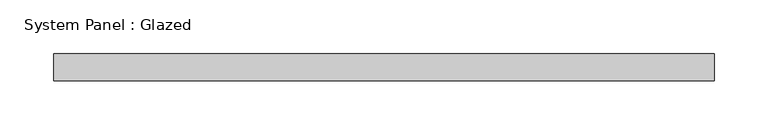
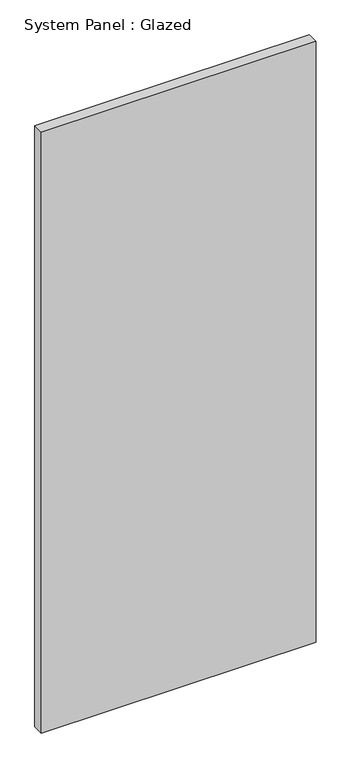
"""IFC4 building model written with IfcOpenShell, lengths in millimetres: plate geometry, System Panel : Glazed."""

from ifc_helpers import new_model, si_unit, origin, origin_with_axes, place, context, project, spatial, polyline, outline, extrude, source, transform, mapped, element, save


def system_panel_glazed_6c2109f1(model_context):
    return source(origin(), model_context, "Body", "SweptSolid", [
        extrude(outline(polyline([(307.975, 19.05), (-307.975, 19.05), (-307.975, 44.45), (307.975, 44.45), (307.975, 19.05)])), origin_with_axes(), (0.0, 0.0, 1.0), 1422.4),
    ])


if __name__ == "__main__":
    model = new_model("IFC4")
    model_context = context("Model", 3, world=origin())
    ifc_project = project(units=[si_unit("LENGTHUNIT", "METRE", prefix="MILLI")], contexts=[model_context])
    site = spatial("IfcSite", under=ifc_project)
    building = spatial("IfcBuilding", under=site)
    placement = place(None, origin())
    system_panel_glazed_shape = system_panel_glazed_6c2109f1(model_context)
    element("IfcPlate", 1, ObjectType="System Panel : Glazed", at=placement, inside=building, context=model_context, shape_type="MappedRepresentation", body=[
        mapped(system_panel_glazed_shape, transform((0.0, 0.0, 0.0), x_axis=(1.0, 0.0, 0.0), y_axis=(0.0, 1.0, 0.0), z_axis=(0.0, 0.0, 1.0))),
    ])
    save(model, "model.ifc")

# Revit data of these elements
# Type "System Panel : Glazed"
#   Construction Type Id = "GSP4R"
#   Analytic Construction = "1/8 in Pilkington single glazing"
#   Visual Light Transmittance = 0.9
#   Solar Heat Gain Coefficient = 0.86
#   Heat Transfer Coefficient (U) = 1.18115 BTU/(h·ft²·°F)
#   Define Thermal Properties by = 1
# Element 1 (IfcPlate, "System Panel : Glazed")
#   Materials on its faces: "Glass"
# Materials
#   "Glass": class "Glass", colour RGB 0 128 192, transparency 0.75, Description = "Soda Lime Glass", Cost = 0
